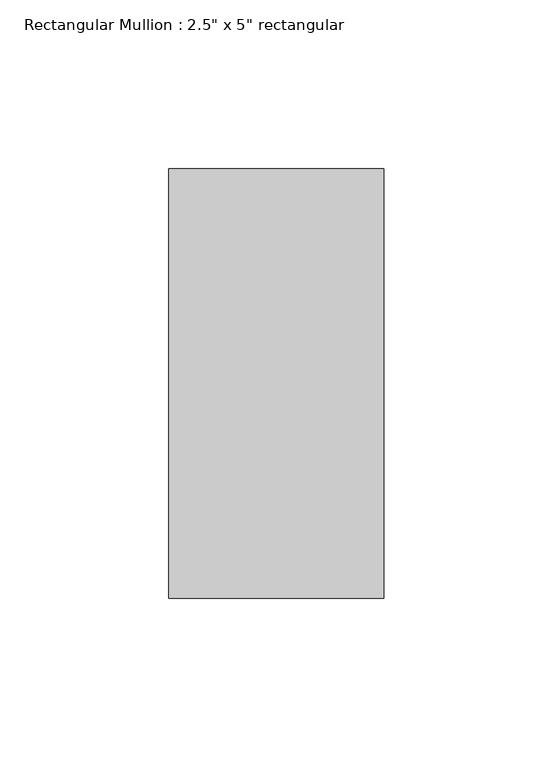
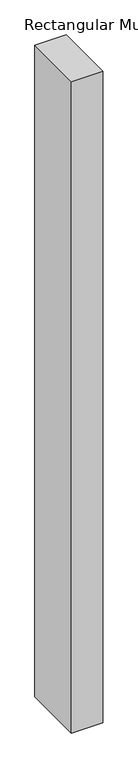
"""IFC4 building model written with IfcOpenShell, lengths in millimetres: member geometry."""

from ifc_helpers import new_model, si_unit, frame, origin, place, context, project, spatial, polyline, outline, extrude, source, transform, mapped, element, save


def member_6a2a75bf(model_context):
    return source(origin(), model_context, "Body", "SweptSolid", [
        extrude(outline(polyline([(0.0, 63.5), (0.0, -63.5), (-63.5, -63.5), (-63.5, 63.5), (0.0, 63.5)])), frame((0.0, 0.0, -1384.7839289), z_axis=(0.0, 0.0, 1.0), x_axis=(1.0, 0.0, 0.0)), (0.0, 0.0, 1.0), 1384.7839289),
    ])


if __name__ == "__main__":
    model = new_model("IFC4")
    model_context = context("Model", 3, world=origin())
    ifc_project = project(units=[si_unit("LENGTHUNIT", "METRE", prefix="MILLI")], contexts=[model_context])
    site = spatial("IfcSite", under=ifc_project)
    building = spatial("IfcBuilding", under=site)
    placement = place(None, origin())
    member_shape = member_6a2a75bf(model_context)
    element("IfcMember", 1, ObjectType="Rectangular Mullion : 2.5\" x 5\" rectangular", at=placement, inside=building, context=model_context, shape_type="MappedRepresentation", body=[
        mapped(member_shape, transform((0.0, 0.0, 0.0), x_axis=(1.0, 0.0, 0.0), y_axis=(0.0, 1.0, 0.0), z_axis=(0.0, 0.0, 1.0))),
    ])
    save(model, "model.ifc")

# Revit data of these elements
# Type "Rectangular Mullion : 2.5\" x 5\" rectangular"
#   built-in parameter 1007304 = 0.416667 (stored number, unit not read)
#   built-in parameter 1007301 = 0.104167 (stored number, unit not read)
#   built-in parameter 1007300 = 0.104167 (stored number, unit not read)
# Element 1 (IfcMember, "Rectangular Mullion : 2.5\" x 5\" rectangular")
#   Materials on its faces: "Aluminum"
# Materials
#   "Aluminum": class "Metal", colour RGB 247 247 247, transparency 0, Description = "Aluminum 6061", Cost = 0
